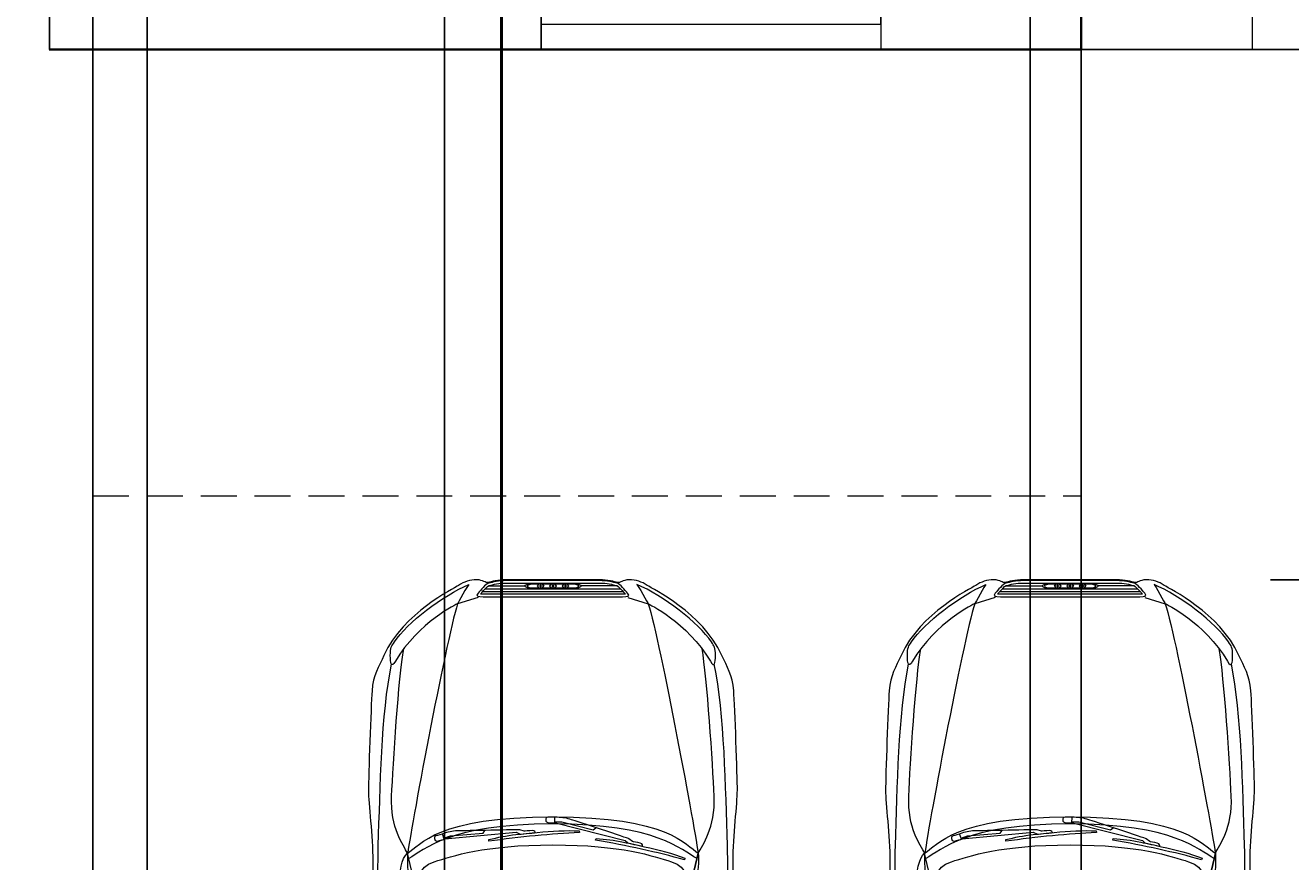
# Model space of a CAD drawing. Units: inches. Extents: x 1770 to 2988, y 1161 to 3221.
# Tile 4 of 44: x 2439 to 2663, y 1467 to 1614. Entities that reach past the tile are written whole.
import ezdxf

# ---------------------------------------------------------------- set-up
doc = ezdxf.new("R2010")
doc.units = ezdxf.units.IN
doc.linetypes.add('DASHED2', pattern=[9.525, 6.35, -3.175])
for name, color, linetype, lineweight in [('A-ANNO-DIMS', 2, 'Continuous', 18), ('A-DOOR', 4, 'Continuous', 18), ('A-GLAZ', 4, 'Continuous', 18), ('A-ROOF-OVHD', 7, 'DASHED2', 18), ('A-WALL', 7, 'Continuous', 35), ('AUDI', 8, 'Continuous', 13), ('C-SITE-PAVE', 8, 'Continuous', 18)]:
    doc.layers.add(name, color=color, linetype=linetype, lineweight=lineweight)
doc.styles.get("Standard").update_dxf_attribs({"font": 'arial.ttf'})
doc.dimstyles.get("Standard").update_dxf_attribs({"dimtxt": 0.18, "dimasz": 0.18, "dimexe": 0.18, "dimexo": 0.0625, "dimgap": 0.09, "dimtad": 0, "dimtih": 1, "dimtoh": 1, "dimdec": 4, "dimzin": 0, "dimdsep": 46, "dimtxsty": 'Standard', "dimcen": 0.09, "dimadec": 0, "dimazin": 0, "dimtfac": 1, "dimtdec": 4, "dimtofl": 0, "dimtmove": 0, "dimatfit": 3, "dimfxl": 1, "dimtolj": 1, "dimtzin": 0, "dimarcsym": 0})

# ---------------------------------------------------------------- blocks, each defined once
blk = doc.blocks.new('CAR-SEDAN-PLAN')
for points, knots in [([(35.35, 0), (11.45, 0.26), (7.98, 8.3), (6.52, 13.59), (6.52, 13.59), (5.56, 16.72), (4.79, 19.21), (4.41, 20.48), (4.41, 20.48), (4.03, 21.76), (3.2, 25.65), (3.14, 28.9), (3.14, 28.9), (3.07, 32.16), (2.76, 51.56), (2.76, 56.91), (2.76, 56.91), (2.76, 62.27), (2.76, 87.35), (2.76, 90.92), (2.76, 90.92), (2.76, 94.49), (3.52, 108.72), (3.52, 113.25), (3.52, 113.25), (3.52, 117.78), (2.76, 123.46), (2.76, 125.81), (2.76, 125.81), (2.76, 128.17), (3.2, 140.62), (3.39, 143.36), (3.39, 143.36), (3.58, 146.1), (4.61, 147.66), (5.5, 149.61), (5.5, 149.61), (8.94, 157.2), (17.74, 161.35), (18.69, 161.99), (18.69, 161.99), (19.65, 162.63), (20.67, 162.97), (21.88, 162.97), (21.88, 162.97), (23.1, 162.97), (23.41, 162.37), (23.92, 162.5), (23.92, 162.5), (24.43, 162.63), (25.7, 162.97), (27.11, 162.97), (27.11, 162.97), (28.52, 162.97), (35.35, 162.97), (35.35, 162.97), (35.35, 162.97), (35.35, 162.97), (42.18, 162.97), (43.59, 162.97), (43.59, 162.97), (45, 162.97), (46.27, 162.63), (46.78, 162.5), (46.78, 162.5), (47.29, 162.37), (47.6, 162.97), (48.82, 162.97), (48.82, 162.97), (50.04, 162.97), (51.05, 162.63), (52.01, 161.99), (52.01, 161.99), (52.96, 161.35), (61.76, 157.2), (65.21, 149.61), (65.21, 149.61), (66.09, 147.66), (67.12, 146.1), (67.31, 143.36), (67.31, 143.36), (67.5, 140.62), (67.95, 128.17), (67.95, 125.81), (67.95, 125.81), (67.95, 123.46), (67.18, 117.78), (67.18, 113.25), (67.18, 113.25), (67.18, 108.72), (67.95, 94.49), (67.95, 90.92), (67.95, 90.92), (67.95, 87.35), (67.95, 62.27), (67.95, 56.91), (67.95, 56.91), (67.95, 51.56), (67.63, 32.16), (67.57, 28.9), (67.57, 28.9), (67.5, 25.65), (66.67, 21.76), (66.29, 20.48), (66.29, 20.48), (65.91, 19.21), (65.14, 16.72), (64.19, 13.59), (64.19, 13.59), (62.72, 8.3), (59.25, 0.26), (35.35, 0)], [0, 0, 0, 0, 0.035714, 0.035714, 0.035714, 0.035714, 0.071429, 0.071429, 0.071429, 0.071429, 0.107143, 0.107143, 0.107143, 0.107143, 0.142857, 0.142857, 0.142857, 0.142857, 0.178571, 0.178571, 0.178571, 0.178571, 0.214286, 0.214286, 0.214286, 0.214286, 0.25, 0.25, 0.25, 0.25, 0.285714, 0.285714, 0.285714, 0.285714, 0.321429, 0.321429, 0.321429, 0.321429, 0.357143, 0.357143, 0.357143, 0.357143, 0.392857, 0.392857, 0.392857, 0.392857, 0.428571, 0.428571, 0.428571, 0.428571, 0.464286, 0.464286, 0.464286, 0.464286, 0.5, 0.5, 0.5, 0.5, 0.535714, 0.535714, 0.535714, 0.535714, 0.571429, 0.571429, 0.571429, 0.571429, 0.607143, 0.607143, 0.607143, 0.607143, 0.642857, 0.642857, 0.642857, 0.642857, 0.678571, 0.678571, 0.678571, 0.678571, 0.714286, 0.714286, 0.714286, 0.714286, 0.75, 0.75, 0.75, 0.75, 0.785714, 0.785714, 0.785714, 0.785714, 0.821429, 0.821429, 0.821429, 0.821429, 0.857143, 0.857143, 0.857143, 0.857143, 0.892857, 0.892857, 0.892857, 0.892857, 0.928571, 0.928571, 0.928571, 0.928571, 0.964286, 0.964286, 0.964286, 0.964286, 1, 1, 1, 1]), ([(6.62, 149.63), (6.62, 148.21), (6.78, 147.35), (7.51, 148.58), (7.51, 148.58), (11.6, 155.5), (18.51, 158.75), (18.51, 158.75), (18.51, 158.75), (18.51, 158.75), (20.38, 162.11), (20.5, 162.15), (20.5, 162.15), (15.94, 160.22), (9.53, 155.36), (7.35, 151.99), (7.35, 151.99), (6.83, 151.3), (6.62, 150.96), (6.62, 149.63)], [0, 0, 0, 0, 0.2, 0.2, 0.2, 0.2, 0.4, 0.4, 0.4, 0.4, 0.6, 0.6, 0.6, 0.6, 0.8, 0.8, 0.8, 0.8, 1, 1, 1, 1]), ([(6.62, 149.63), (6.62, 148.21), (6.78, 147.35), (7.51, 148.58), (7.51, 148.58), (11.6, 155.5), (18.51, 158.75), (18.51, 158.75), (18.51, 158.75), (18.51, 158.75), (20.38, 162.11), (20.5, 162.15), (20.5, 162.15), (15.94, 160.22), (9.53, 155.36), (7.35, 151.99), (7.35, 151.99), (6.83, 151.3), (6.62, 150.96), (6.62, 149.63)], [0, 0, 0, 0, 0.2, 0.2, 0.2, 0.2, 0.4, 0.4, 0.4, 0.4, 0.6, 0.6, 0.6, 0.6, 0.8, 0.8, 0.8, 0.8, 1, 1, 1, 1]), ([(35.49, 162.83), (35.49, 162.83), (43.59, 162.83), (43.59, 162.83), (43.59, 162.83), (44.89, 162.83), (46.07, 162.53), (46.64, 162.39), (46.64, 162.39), (46.64, 162.39), (46.74, 162.36), (46.74, 162.36), (46.74, 162.36), (47.26, 162.2), (48.06, 161.16), (48.56, 160.6), (48.56, 160.6), (49.07, 160.04), (48.56, 159.99), (47.66, 159.99), (47.66, 159.99), (46.75, 159.99), (35.35, 159.99), (35.35, 159.99), (35.35, 159.99), (35.35, 159.99), (23.95, 159.99), (23.04, 159.99), (23.04, 159.99), (22.14, 159.99), (21.63, 160.04), (22.14, 160.6), (22.14, 160.6), (22.64, 161.16), (23.44, 162.2), (23.96, 162.36), (23.96, 162.36), (23.96, 162.36), (24.06, 162.39), (24.06, 162.39), (24.06, 162.39), (24.63, 162.53), (25.81, 162.83), (27.11, 162.83), (27.11, 162.83), (27.11, 162.83), (35.22, 162.83), (35.22, 162.83), (35.22, 162.83), (35.22, 162.83), (35.49, 162.83), (35.49, 162.83)], [0, 0, 0, 0, 0.076923, 0.076923, 0.076923, 0.076923, 0.153846, 0.153846, 0.153846, 0.153846, 0.230769, 0.230769, 0.230769, 0.230769, 0.307692, 0.307692, 0.307692, 0.307692, 0.384615, 0.384615, 0.384615, 0.384615, 0.461538, 0.461538, 0.461538, 0.461538, 0.538462, 0.538462, 0.538462, 0.538462, 0.615385, 0.615385, 0.615385, 0.615385, 0.692308, 0.692308, 0.692308, 0.692308, 0.769231, 0.769231, 0.769231, 0.769231, 0.846154, 0.846154, 0.846154, 0.846154, 0.923077, 0.923077, 0.923077, 0.923077, 1, 1, 1, 1]), ([(23.04, 160.41), (23.04, 160.41), (23.04, 160.41), (23.04, 160.41), (23.04, 160.41), (23.04, 160.41), (47.66, 160.41), (47.66, 160.41), (47.66, 160.41), (47.87, 160.41), (48.03, 160.42), (48.16, 160.43), (48.16, 160.43), (48.06, 160.54), (47.9, 160.72), (47.9, 160.72), (47.9, 160.72), (47.53, 161.15), (46.91, 161.87), (46.62, 161.96), (46.62, 161.96), (46.62, 161.96), (46.53, 161.98), (46.53, 161.98), (46.53, 161.98), (45.98, 162.12), (44.84, 162.41), (43.59, 162.41), (43.59, 162.41), (43.59, 162.41), (27.11, 162.41), (27.11, 162.41), (27.11, 162.41), (25.87, 162.41), (24.72, 162.12), (24.17, 161.98), (24.17, 161.98), (24.17, 161.98), (24.06, 161.95), (24.06, 161.95), (24.06, 161.95), (23.79, 161.87), (23.17, 161.15), (22.8, 160.72), (22.8, 160.72), (22.8, 160.72), (22.65, 160.54), (22.55, 160.43), (22.55, 160.43), (22.68, 160.42), (22.84, 160.41), (23.04, 160.41)], [0, 0, 0, 0, 0.076923, 0.076923, 0.076923, 0.076923, 0.153846, 0.153846, 0.153846, 0.153846, 0.230769, 0.230769, 0.230769, 0.230769, 0.307692, 0.307692, 0.307692, 0.307692, 0.384615, 0.384615, 0.384615, 0.384615, 0.461538, 0.461538, 0.461538, 0.461538, 0.538462, 0.538462, 0.538462, 0.538462, 0.615385, 0.615385, 0.615385, 0.615385, 0.692308, 0.692308, 0.692308, 0.692308, 0.769231, 0.769231, 0.769231, 0.769231, 0.846154, 0.846154, 0.846154, 0.846154, 0.923077, 0.923077, 0.923077, 0.923077, 1, 1, 1, 1]), ([(32.06, 161.44), (32.49, 161.44), (32.87, 161.48), (33.16, 161.56), (33.16, 161.56), (33.46, 161.48), (33.86, 161.44), (34.29, 161.44), (34.29, 161.44), (34.72, 161.44), (35.09, 161.48), (35.39, 161.55), (35.39, 161.55), (35.65, 161.48), (36.06, 161.44), (36.46, 161.44), (36.46, 161.44), (36.89, 161.44), (37.29, 161.48), (37.58, 161.56), (37.58, 161.56), (37.88, 161.48), (38.25, 161.44), (38.68, 161.44), (38.68, 161.44), (39.59, 161.44), (40.34, 161.64), (40.34, 161.88), (40.34, 161.88), (40.34, 162.12), (39.59, 162.32), (38.68, 162.32), (38.68, 162.32), (38.25, 162.32), (37.88, 162.27), (37.58, 162.21), (37.58, 162.21), (37.29, 162.27), (36.89, 162.32), (36.46, 162.32), (36.46, 162.32), (36.06, 162.32), (35.65, 162.28), (35.39, 162.21), (35.39, 162.21), (35.09, 162.28), (34.72, 162.32), (34.29, 162.32), (34.29, 162.32), (33.81, 162.32), (33.29, 162.24), (33.16, 162.21), (33.16, 162.21), (32.87, 162.27), (32.49, 162.32), (32.06, 162.32), (32.06, 162.32), (31.15, 162.32), (30.4, 162.12), (30.4, 161.88), (30.4, 161.88), (30.4, 161.64), (31.15, 161.44), (32.06, 161.44)], [0, 0, 0, 0, 0.0625, 0.0625, 0.0625, 0.0625, 0.125, 0.125, 0.125, 0.125, 0.1875, 0.1875, 0.1875, 0.1875, 0.25, 0.25, 0.25, 0.25, 0.3125, 0.3125, 0.3125, 0.3125, 0.375, 0.375, 0.375, 0.375, 0.4375, 0.4375, 0.4375, 0.4375, 0.5, 0.5, 0.5, 0.5, 0.5625, 0.5625, 0.5625, 0.5625, 0.625, 0.625, 0.625, 0.625, 0.6875, 0.6875, 0.6875, 0.6875, 0.75, 0.75, 0.75, 0.75, 0.8125, 0.8125, 0.8125, 0.8125, 0.875, 0.875, 0.875, 0.875, 0.9375, 0.9375, 0.9375, 0.9375, 1, 1, 1, 1]), ([(32.06, 161.44), (32.49, 161.44), (32.87, 161.48), (33.16, 161.56), (33.16, 161.56), (33.46, 161.48), (33.86, 161.44), (34.29, 161.44), (34.29, 161.44), (34.72, 161.44), (35.09, 161.48), (35.39, 161.55), (35.39, 161.55), (35.65, 161.48), (36.06, 161.44), (36.46, 161.44), (36.46, 161.44), (36.89, 161.44), (37.29, 161.48), (37.58, 161.56), (37.58, 161.56), (37.88, 161.48), (38.25, 161.44), (38.68, 161.44), (38.68, 161.44), (39.59, 161.44), (40.34, 161.64), (40.34, 161.88), (40.34, 161.88), (40.34, 162.12), (39.59, 162.32), (38.68, 162.32), (38.68, 162.32), (38.25, 162.32), (37.88, 162.27), (37.58, 162.21), (37.58, 162.21), (37.29, 162.27), (36.89, 162.32), (36.46, 162.32), (36.46, 162.32), (36.06, 162.32), (35.65, 162.28), (35.39, 162.21), (35.39, 162.21), (35.09, 162.28), (34.72, 162.32), (34.29, 162.32), (34.29, 162.32), (33.81, 162.32), (33.29, 162.24), (33.16, 162.21), (33.16, 162.21), (32.87, 162.27), (32.49, 162.32), (32.06, 162.32), (32.06, 162.32), (31.15, 162.32), (30.4, 162.12), (30.4, 161.88), (30.4, 161.88), (30.4, 161.64), (31.15, 161.44), (32.06, 161.44)], [0, 0, 0, 0, 0.0625, 0.0625, 0.0625, 0.0625, 0.125, 0.125, 0.125, 0.125, 0.1875, 0.1875, 0.1875, 0.1875, 0.25, 0.25, 0.25, 0.25, 0.3125, 0.3125, 0.3125, 0.3125, 0.375, 0.375, 0.375, 0.375, 0.4375, 0.4375, 0.4375, 0.4375, 0.5, 0.5, 0.5, 0.5, 0.5625, 0.5625, 0.5625, 0.5625, 0.625, 0.625, 0.625, 0.625, 0.6875, 0.6875, 0.6875, 0.6875, 0.75, 0.75, 0.75, 0.75, 0.8125, 0.8125, 0.8125, 0.8125, 0.875, 0.875, 0.875, 0.875, 0.9375, 0.9375, 0.9375, 0.9375, 1, 1, 1, 1]), ([(32.06, 162.21), (32.39, 162.21), (32.68, 162.18), (32.89, 162.12), (32.89, 162.12), (32.73, 162.05), (32.63, 161.97), (32.63, 161.88), (32.63, 161.88), (32.63, 161.79), (32.73, 161.71), (32.89, 161.64), (32.89, 161.64), (32.68, 161.59), (32.39, 161.55), (32.06, 161.55), (32.06, 161.55), (31.37, 161.55), (30.83, 161.69), (30.83, 161.88), (30.83, 161.88), (30.83, 162.06), (31.37, 162.21), (32.06, 162.21)], [0, 0, 0, 0, 0.166667, 0.166667, 0.166667, 0.166667, 0.333333, 0.333333, 0.333333, 0.333333, 0.5, 0.5, 0.5, 0.5, 0.666667, 0.666667, 0.666667, 0.666667, 0.833333, 0.833333, 0.833333, 0.833333, 1, 1, 1, 1]), ([(33.3, 161.88), (33.3, 161.82), (33.24, 161.78), (33.16, 161.74), (33.16, 161.74), (33.08, 161.78), (33.06, 161.82), (33.06, 161.88), (33.06, 161.88), (33.06, 161.93), (33.08, 161.98), (33.16, 162.03), (33.16, 162.03), (33.24, 161.98), (33.3, 161.93), (33.3, 161.88)], [0, 0, 0, 0, 0.25, 0.25, 0.25, 0.25, 0.5, 0.5, 0.5, 0.5, 0.75, 0.75, 0.75, 0.75, 1, 1, 1, 1]), ([(35.09, 162.13), (34.93, 162.06), (34.82, 161.97), (34.82, 161.88), (34.82, 161.88), (34.82, 161.79), (34.93, 161.7), (35.09, 161.63), (35.09, 161.63), (34.88, 161.58), (34.61, 161.55), (34.29, 161.55), (34.29, 161.55), (33.97, 161.55), (33.67, 161.59), (33.46, 161.64), (33.46, 161.64), (33.62, 161.71), (33.73, 161.79), (33.73, 161.88), (33.73, 161.88), (33.73, 161.97), (33.62, 162.05), (33.46, 162.12), (33.46, 162.12), (33.67, 162.18), (33.97, 162.21), (34.29, 162.21), (34.29, 162.21), (34.61, 162.21), (34.88, 162.18), (35.09, 162.13)], [0, 0, 0, 0, 0.125, 0.125, 0.125, 0.125, 0.25, 0.25, 0.25, 0.25, 0.375, 0.375, 0.375, 0.375, 0.5, 0.5, 0.5, 0.5, 0.625, 0.625, 0.625, 0.625, 0.75, 0.75, 0.75, 0.75, 0.875, 0.875, 0.875, 0.875, 1, 1, 1, 1]), ([(35.52, 161.88), (35.52, 161.82), (35.47, 161.77), (35.39, 161.72), (35.39, 161.72), (35.28, 161.77), (35.23, 161.82), (35.23, 161.88), (35.23, 161.88), (35.23, 161.93), (35.28, 161.99), (35.39, 162.03), (35.39, 162.03), (35.47, 161.99), (35.52, 161.93), (35.52, 161.88)], [0, 0, 0, 0, 0.25, 0.25, 0.25, 0.25, 0.5, 0.5, 0.5, 0.5, 0.75, 0.75, 0.75, 0.75, 1, 1, 1, 1]), ([(37.32, 162.12), (37.13, 162.05), (37.02, 161.97), (37.02, 161.88), (37.02, 161.88), (37.02, 161.79), (37.13, 161.71), (37.32, 161.64), (37.32, 161.64), (37.07, 161.59), (36.78, 161.55), (36.46, 161.55), (36.46, 161.55), (36.16, 161.55), (35.87, 161.58), (35.65, 161.63), (35.65, 161.63), (35.84, 161.7), (35.95, 161.79), (35.95, 161.88), (35.95, 161.88), (35.95, 161.97), (35.84, 162.06), (35.65, 162.13), (35.65, 162.13), (35.87, 162.18), (36.16, 162.21), (36.46, 162.21), (36.46, 162.21), (36.78, 162.21), (37.07, 162.18), (37.32, 162.12)], [0, 0, 0, 0, 0.125, 0.125, 0.125, 0.125, 0.25, 0.25, 0.25, 0.25, 0.375, 0.375, 0.375, 0.375, 0.5, 0.5, 0.5, 0.5, 0.625, 0.625, 0.625, 0.625, 0.75, 0.75, 0.75, 0.75, 0.875, 0.875, 0.875, 0.875, 1, 1, 1, 1]), ([(37.72, 161.88), (37.72, 161.82), (37.66, 161.78), (37.58, 161.74), (37.58, 161.74), (37.5, 161.78), (37.45, 161.82), (37.45, 161.88), (37.45, 161.88), (37.45, 161.93), (37.5, 161.98), (37.58, 162.03), (37.58, 162.03), (37.66, 161.98), (37.72, 161.93), (37.72, 161.88)], [0, 0, 0, 0, 0.25, 0.25, 0.25, 0.25, 0.5, 0.5, 0.5, 0.5, 0.75, 0.75, 0.75, 0.75, 1, 1, 1, 1]), ([(39.91, 161.88), (39.91, 161.69), (39.38, 161.55), (38.68, 161.55), (38.68, 161.55), (38.36, 161.55), (38.07, 161.59), (37.85, 161.64), (37.85, 161.64), (38.01, 161.71), (38.12, 161.79), (38.12, 161.88), (38.12, 161.88), (38.12, 161.97), (38.01, 162.05), (37.85, 162.12), (37.85, 162.12), (38.07, 162.18), (38.36, 162.21), (38.68, 162.21), (38.68, 162.21), (39.38, 162.21), (39.91, 162.06), (39.91, 161.88)], [0, 0, 0, 0, 0.166667, 0.166667, 0.166667, 0.166667, 0.333333, 0.333333, 0.333333, 0.333333, 0.5, 0.5, 0.5, 0.5, 0.666667, 0.666667, 0.666667, 0.666667, 0.833333, 0.833333, 0.833333, 0.833333, 1, 1, 1, 1]), ([(64.08, 149.63), (64.08, 148.21), (63.92, 147.35), (63.19, 148.58), (63.19, 148.58), (59.11, 155.5), (52.19, 158.75), (52.19, 158.75), (52.19, 158.75), (52.19, 158.75), (50.32, 162.11), (50.2, 162.15), (50.2, 162.15), (54.76, 160.22), (61.17, 155.36), (63.35, 151.99), (63.35, 151.99), (63.87, 151.3), (64.08, 150.96), (64.08, 149.63)], [0, 0, 0, 0, 0.2, 0.2, 0.2, 0.2, 0.4, 0.4, 0.4, 0.4, 0.6, 0.6, 0.6, 0.6, 0.8, 0.8, 0.8, 0.8, 1, 1, 1, 1]), ([(64.08, 149.63), (64.08, 148.21), (63.92, 147.35), (63.19, 148.58), (63.19, 148.58), (59.11, 155.5), (52.19, 158.75), (52.19, 158.75), (52.19, 158.75), (52.19, 158.75), (50.32, 162.11), (50.2, 162.15), (50.2, 162.15), (54.76, 160.22), (61.17, 155.36), (63.35, 151.99), (63.35, 151.99), (63.87, 151.3), (64.08, 150.96), (64.08, 149.63)], [0, 0, 0, 0, 0.2, 0.2, 0.2, 0.2, 0.4, 0.4, 0.4, 0.4, 0.6, 0.6, 0.6, 0.6, 0.8, 0.8, 0.8, 0.8, 1, 1, 1, 1]), ([(9.66, 114.67), (8.92, 116.16), (6.61, 119.13), (6.86, 124.74), (6.86, 124.74), (7.1, 130.36), (8.1, 145.86), (8.99, 150.79)], [0, 0, 0, 0, 0.5, 0.5, 0.5, 0.5, 1, 1, 1, 1]), ([(61.04, 114.67), (61.78, 116.16), (64.09, 119.13), (63.85, 124.74), (63.85, 124.74), (63.6, 130.36), (62.6, 145.86), (61.71, 150.79)], [0, 0, 0, 0, 0.5, 0.5, 0.5, 0.5, 1, 1, 1, 1]), ([(7.64, 13.52), (6.44, 19.53), (5.16, 31.7), (4.94, 44.37), (4.94, 44.37), (4.72, 57.04), (4.17, 105.75), (4.5, 116.02), (4.5, 116.02), (4.83, 126.28), (5.01, 139.24), (6.83, 148.05)], [0, 0, 0, 0, 0.333333, 0.333333, 0.333333, 0.333333, 0.666667, 0.666667, 0.666667, 0.666667, 1, 1, 1, 1]), ([(63.07, 13.52), (64.27, 19.53), (65.54, 31.7), (65.76, 44.37), (65.76, 44.37), (65.98, 57.04), (66.53, 105.75), (66.2, 116.02), (66.2, 116.02), (65.87, 126.28), (65.69, 139.24), (63.87, 148.05)], [0, 0, 0, 0, 0.333333, 0.333333, 0.333333, 0.333333, 0.666667, 0.666667, 0.666667, 0.666667, 1, 1, 1, 1]), ([(35.35, 92.33), (46.17, 92.33), (55.33, 90.37), (55.33, 90.37), (55.33, 90.37), (55.33, 90.37), (61.04, 114.67), (61.04, 114.67), (61.04, 114.67), (58.76, 116.14), (55.78, 121.11), (35.35, 121.11), (35.35, 121.11), (14.92, 121.11), (11.94, 116.14), (9.66, 114.67), (9.66, 114.67), (9.66, 114.67), (15.37, 90.37), (15.37, 90.37), (15.37, 90.37), (15.37, 90.37), (24.53, 92.33), (35.35, 92.33)], [0, 0, 0, 0, 0.166667, 0.166667, 0.166667, 0.166667, 0.333333, 0.333333, 0.333333, 0.333333, 0.5, 0.5, 0.5, 0.5, 0.666667, 0.666667, 0.666667, 0.666667, 0.833333, 0.833333, 0.833333, 0.833333, 1, 1, 1, 1]), ([(35.35, 92.33), (46.17, 92.33), (55.33, 90.37), (55.33, 90.37), (55.33, 90.37), (55.33, 90.37), (61.04, 114.67), (61.04, 114.67), (61.04, 114.67), (58.76, 116.14), (55.78, 121.11), (35.35, 121.11), (35.35, 121.11), (14.92, 121.11), (11.94, 116.14), (9.66, 114.67), (9.66, 114.67), (9.66, 114.67), (15.37, 90.37), (15.37, 90.37), (15.37, 90.37), (15.37, 90.37), (24.53, 92.33), (35.35, 92.33)], [0, 0, 0, 0, 0.166667, 0.166667, 0.166667, 0.166667, 0.333333, 0.333333, 0.333333, 0.333333, 0.5, 0.5, 0.5, 0.5, 0.666667, 0.666667, 0.666667, 0.666667, 0.833333, 0.833333, 0.833333, 0.833333, 1, 1, 1, 1]), ([(36.09, 121.02), (37.08, 121.02), (37.81, 120.86), (38.66, 120.59), (38.66, 120.59), (39.31, 120.41), (48.79, 117.24), (48.79, 117.24), (48.79, 117.24), (48.79, 117.24), (49.43, 116.73), (49.43, 116.73), (49.43, 116.73), (49.43, 116.73), (50.29, 116.57), (50.77, 116.47), (50.77, 116.47), (51.26, 116.33), (51.2, 115.9), (51.2, 115.9), (51.2, 115.9), (51.2, 115.9), (48.58, 116.49), (48.58, 116.49), (48.58, 116.49), (48.58, 116.49), (48.15, 116.92), (48.15, 116.92), (48.15, 116.92), (48.15, 116.92), (35.82, 120.06), (35.82, 120.06), (35.82, 120.06), (35.82, 120.06), (35.42, 120.06), (34.8, 120.06), (34.8, 120.06), (34.19, 120.09), (34.08, 120.3), (34.08, 120.54), (34.08, 120.54), (34.08, 120.81), (34.11, 121.05), (34.48, 121.05), (34.48, 121.05), (34.86, 121.08), (35.47, 121.05), (36.09, 121.02)], [0, 0, 0, 0, 0.083333, 0.083333, 0.083333, 0.083333, 0.166667, 0.166667, 0.166667, 0.166667, 0.25, 0.25, 0.25, 0.25, 0.333333, 0.333333, 0.333333, 0.333333, 0.416667, 0.416667, 0.416667, 0.416667, 0.5, 0.5, 0.5, 0.5, 0.583333, 0.583333, 0.583333, 0.583333, 0.666667, 0.666667, 0.666667, 0.666667, 0.75, 0.75, 0.75, 0.75, 0.833333, 0.833333, 0.833333, 0.833333, 0.916667, 0.916667, 0.916667, 0.916667, 1, 1, 1, 1]), ([(60.82, 113.75), (58.05, 115.23), (53.75, 119.85), (35.35, 119.85), (35.35, 119.85), (16.95, 119.85), (12.66, 115.23), (9.88, 113.75)], [0, 0, 0, 0, 0.5, 0.5, 0.5, 0.5, 1, 1, 1, 1]), ([(16.21, 118.21), (17.12, 118.53), (17.87, 118.61), (18.78, 118.64), (18.78, 118.64), (19.45, 118.64), (29.53, 118.83), (29.53, 118.83), (29.53, 118.83), (29.53, 118.83), (30.3, 118.56), (30.3, 118.56), (30.3, 118.56), (30.3, 118.56), (31.19, 118.66), (31.67, 118.69), (31.67, 118.69), (32.15, 118.75), (32.23, 118.32), (32.23, 118.32), (32.23, 118.32), (32.23, 118.32), (29.58, 118.05), (29.58, 118.05), (29.58, 118.05), (29.58, 118.05), (28.86, 118.4), (28.86, 118.4), (28.86, 118.4), (28.86, 118.4), (16.26, 117.22), (16.26, 117.22), (16.26, 117.22), (16.26, 117.22), (15.89, 117.08), (15.3, 116.9), (15.3, 116.9), (14.74, 116.71), (14.55, 116.87), (14.47, 117.11), (14.47, 117.11), (14.39, 117.38), (14.33, 117.59), (14.68, 117.73), (14.68, 117.73), (15.03, 117.83), (15.62, 118.02), (16.21, 118.21)], [0, 0, 0, 0, 0.083333, 0.083333, 0.083333, 0.083333, 0.166667, 0.166667, 0.166667, 0.166667, 0.25, 0.25, 0.25, 0.25, 0.333333, 0.333333, 0.333333, 0.333333, 0.416667, 0.416667, 0.416667, 0.416667, 0.5, 0.5, 0.5, 0.5, 0.583333, 0.583333, 0.583333, 0.583333, 0.666667, 0.666667, 0.666667, 0.666667, 0.75, 0.75, 0.75, 0.75, 0.833333, 0.833333, 0.833333, 0.833333, 0.916667, 0.916667, 0.916667, 0.916667, 1, 1, 1, 1]), ([(16.21, 118.21), (17.12, 118.53), (17.87, 118.61), (18.78, 118.64), (18.78, 118.64), (19.45, 118.64), (29.53, 118.83), (29.53, 118.83), (29.53, 118.83), (29.53, 118.83), (30.3, 118.56), (30.3, 118.56), (30.3, 118.56), (30.3, 118.56), (31.19, 118.66), (31.67, 118.69), (31.67, 118.69), (32.15, 118.75), (32.23, 118.32), (32.23, 118.32), (32.23, 118.32), (32.23, 118.32), (29.58, 118.05), (29.58, 118.05), (29.58, 118.05), (29.58, 118.05), (28.86, 118.4), (28.86, 118.4), (28.86, 118.4), (28.86, 118.4), (16.26, 117.22), (16.26, 117.22), (16.26, 117.22), (16.26, 117.22), (15.89, 117.08), (15.3, 116.9), (15.3, 116.9), (14.74, 116.71), (14.55, 116.87), (14.47, 117.11), (14.47, 117.11), (14.39, 117.38), (14.33, 117.59), (14.68, 117.73), (14.68, 117.73), (15.03, 117.83), (15.62, 118.02), (16.21, 118.21)], [0, 0, 0, 0, 0.083333, 0.083333, 0.083333, 0.083333, 0.166667, 0.166667, 0.166667, 0.166667, 0.25, 0.25, 0.25, 0.25, 0.333333, 0.333333, 0.333333, 0.333333, 0.416667, 0.416667, 0.416667, 0.416667, 0.5, 0.5, 0.5, 0.5, 0.583333, 0.583333, 0.583333, 0.583333, 0.666667, 0.666667, 0.666667, 0.666667, 0.75, 0.75, 0.75, 0.75, 0.833333, 0.833333, 0.833333, 0.833333, 0.916667, 0.916667, 0.916667, 0.916667, 1, 1, 1, 1]), ([(16.1, 117.35), (16.1, 117.35), (17.26, 117.73), (17.26, 117.73), (17.26, 117.73), (17.26, 117.73), (23.02, 118.24), (23.02, 118.24), (23.02, 118.24), (23.02, 118.24), (23.34, 118.69), (23.34, 118.69)], [0, 0, 0, 0, 0.333333, 0.333333, 0.333333, 0.333333, 0.666667, 0.666667, 0.666667, 0.666667, 1, 1, 1, 1]), ([(40, 118.61), (37.7, 118.77), (35.18, 118.58), (32.58, 118.34), (32.58, 118.34), (31.32, 118.21), (30.06, 118.1), (28.83, 117.97), (28.83, 117.97), (27.09, 117.81), (25.61, 117.46), (24.01, 117.08), (24.01, 117.08), (24.01, 117.08), (24.01, 116.79), (24.01, 116.79), (24.01, 116.79), (29.47, 117.57), (35.15, 118.1), (40.03, 118.32), (40.03, 118.32), (40.03, 118.32), (40, 118.61), (40, 118.61)], [0, 0, 0, 0, 0.166667, 0.166667, 0.166667, 0.166667, 0.333333, 0.333333, 0.333333, 0.333333, 0.5, 0.5, 0.5, 0.5, 0.666667, 0.666667, 0.666667, 0.666667, 0.833333, 0.833333, 0.833333, 0.833333, 1, 1, 1, 1]), ([(35.69, 120.25), (35.69, 120.25), (36.92, 120.22), (36.92, 120.22), (36.92, 120.22), (36.92, 120.22), (42.49, 118.83), (42.49, 118.83), (42.49, 118.83), (42.49, 118.83), (42.95, 119.17), (42.95, 119.17)], [0, 0, 0, 0, 0.333333, 0.333333, 0.333333, 0.333333, 0.666667, 0.666667, 0.666667, 0.666667, 1, 1, 1, 1]), ([(58.68, 113.81), (56.53, 114.64), (54.1, 115.26), (51.52, 115.82), (51.52, 115.82), (50.29, 116.09), (49.06, 116.39), (47.85, 116.63), (47.85, 116.63), (46.17, 117), (44.64, 117.14), (42.98, 117.27), (42.98, 117.27), (42.98, 117.27), (42.9, 117), (42.9, 117), (42.9, 117), (48.34, 116.06), (53.88, 114.83), (58.6, 113.52), (58.6, 113.52), (58.6, 113.52), (58.68, 113.81), (58.68, 113.81)], [0, 0, 0, 0, 0.166667, 0.166667, 0.166667, 0.166667, 0.333333, 0.333333, 0.333333, 0.333333, 0.5, 0.5, 0.5, 0.5, 0.666667, 0.666667, 0.666667, 0.666667, 0.833333, 0.833333, 0.833333, 0.833333, 1, 1, 1, 1]), ([(9.66, 114.67), (9.66, 114.67), (15.37, 90.37), (15.37, 90.37), (15.37, 90.37), (15.37, 90.37), (14.48, 91.26), (14.15, 92.64), (14.15, 92.64), (13.82, 94.03), (10.04, 109.86), (9.79, 111.17), (9.79, 111.17), (9.55, 112.47), (9.66, 114.67), (9.66, 114.67)], [0, 0, 0, 0, 0.25, 0.25, 0.25, 0.25, 0.5, 0.5, 0.5, 0.5, 0.75, 0.75, 0.75, 0.75, 1, 1, 1, 1]), ([(9.66, 114.67), (9.66, 114.67), (15.37, 90.37), (15.37, 90.37), (15.37, 90.37), (15.37, 90.37), (14.48, 91.26), (14.15, 92.64), (14.15, 92.64), (13.82, 94.03), (10.04, 109.86), (9.79, 111.17), (9.79, 111.17), (9.55, 112.47), (9.66, 114.67), (9.66, 114.67)], [0, 0, 0, 0, 0.25, 0.25, 0.25, 0.25, 0.5, 0.5, 0.5, 0.5, 0.75, 0.75, 0.75, 0.75, 1, 1, 1, 1]), ([(35.35, 93.86), (43.94, 93.86), (50.97, 92.45), (52.59, 92.2), (52.59, 92.2), (53.92, 92), (55.15, 93.44), (55.52, 95.16), (55.52, 95.16), (55.89, 96.88), (58.26, 106.94), (58.59, 108.38), (58.59, 108.38), (58.92, 109.82), (59.47, 112.19), (56.31, 113.17), (56.31, 113.17), (53.15, 114.15), (47.56, 116.15), (35.35, 116.15), (35.35, 116.15), (23.15, 116.15), (17.55, 114.15), (14.39, 113.17), (14.39, 113.17), (11.23, 112.19), (11.79, 109.82), (12.11, 108.38), (12.11, 108.38), (12.44, 106.94), (14.81, 96.88), (15.18, 95.16), (15.18, 95.16), (15.55, 93.44), (16.78, 92), (18.11, 92.2), (18.11, 92.2), (19.74, 92.45), (26.76, 93.86), (35.35, 93.86)], [0, 0, 0, 0, 0.1, 0.1, 0.1, 0.1, 0.2, 0.2, 0.2, 0.2, 0.3, 0.3, 0.3, 0.3, 0.4, 0.4, 0.4, 0.4, 0.5, 0.5, 0.5, 0.5, 0.6, 0.6, 0.6, 0.6, 0.7, 0.7, 0.7, 0.7, 0.8, 0.8, 0.8, 0.8, 0.9, 0.9, 0.9, 0.9, 1, 1, 1, 1]), ([(61.04, 114.67), (61.04, 114.67), (55.33, 90.37), (55.33, 90.37), (55.33, 90.37), (55.33, 90.37), (56.23, 91.26), (56.55, 92.64), (56.55, 92.64), (56.88, 94.03), (60.66, 109.86), (60.91, 111.17), (60.91, 111.17), (61.15, 112.47), (61.04, 114.67), (61.04, 114.67)], [0, 0, 0, 0, 0.25, 0.25, 0.25, 0.25, 0.5, 0.5, 0.5, 0.5, 0.75, 0.75, 0.75, 0.75, 1, 1, 1, 1])]:
    blk.add_open_spline(points, degree=3, knots=knots)
for points in [[(23.41, 161.4), (23.41, 161.4), (47.23, 161.4), (47.23, 161.4)], [(23.96, 161.9), (23.96, 161.9), (30.4, 161.9), (30.4, 161.9)], [(46.75, 161.9), (46.75, 161.9), (40.3, 161.9), (40.3, 161.9)], [(22.13, 159.86), (22.13, 159.86), (18.51, 158.75), (18.51, 158.75)], [(22.94, 160.88), (22.94, 160.88), (47.74, 160.88), (47.74, 160.88)], [(48.57, 159.86), (48.57, 159.86), (52.19, 158.75), (52.19, 158.75)], [(18.51, 158.75), (16.41, 152.05), (10.02, 117.73), (9.65, 114.38)], [(52.19, 158.75), (54.3, 152.05), (60.68, 117.73), (61.05, 114.38)], [(35.69, 120.06), (35.69, 120.06), (35.72, 121.05), (35.72, 121.05)], [(16.16, 117.16), (16.16, 117.16), (15.83, 118.1), (15.83, 118.1)], [(8.16, 109.91), (8.28, 111.03), (8.55, 113.81), (9.66, 114.67)]]:
    blk.add_open_spline(points, degree=3)
blk = doc.blocks.new('WIN-60-EXT')
for p, q in [((0, 9), (0, 0)), ((60, 4.5), (60, 9)), ((60, 9), (60, 0)), ((0, 0), (0, 4.5)), ((0, 4.5), (60, 4.5))]:
    blk.add_line(p, q)
blk = doc.blocks.new('*D50')
at = {"layer": 'A-ANNO-DIMS', "color": 0, "lineweight": -2, "transparency": 16777216}
for p, q in [((2659.16, 1516.52), (2683.72, 1516.52)), ((2683.54, 1516.34), (2683.54, 1435.22)), ((2683.54, 1353.73), (2683.54, 1434.85)), ((2659.16, 1353.55), (2683.72, 1353.55))]:
    blk.add_line(p, q, dxfattribs=at)
at = {"layer": 'A-ANNO-DIMS', "color": 0, "transparency": 16777216}
for points in [[(2683.51, 1516.34), (2683.57, 1516.34), (2683.54, 1516.52)], [(2683.51, 1353.73), (2683.57, 1353.73), (2683.54, 1353.55)]]:
    blk.add_solid(points, dxfattribs=at)
at = {"layer": 'Defpoints', "color": 0, "transparency": 16777216}
for p in [(2659.1, 1516.52), (2683.54, 1516.52), (2659.1, 1353.55)]:
    blk.add_point(p, dxfattribs=at)
at = {"layer": 'A-ANNO-DIMS', "color": 0, "transparency": 16777216, "insert": (2683.54, 1435.04), "char_height": 0.18, "attachment_point": 5}
blk.add_mtext('\\A1;SEDAN 163 TYP.', dxfattribs=at)
blk = doc.blocks.new('*D60')
at = {"layer": 'A-ANNO-DIMS', "color": 0, "lineweight": -2, "transparency": 16777216}
for p, q in [((2151.7, 1610.14), (2151.7, 1165.57)), ((2625.7, 1610.14), (2625.7, 1165.57)), ((2151.88, 1165.75), (2388.4, 1165.75)), ((2625.52, 1165.75), (2388.99, 1165.75))]:
    blk.add_line(p, q, dxfattribs=at)
at = {"layer": 'A-ANNO-DIMS', "color": 0, "transparency": 16777216}
for points in [[(2151.88, 1165.78), (2151.88, 1165.72), (2151.7, 1165.75)], [(2625.52, 1165.78), (2625.52, 1165.72), (2625.7, 1165.75)]]:
    blk.add_solid(points, dxfattribs=at)
at = {"layer": 'Defpoints', "color": 0, "transparency": 16777216}
for p in [(2151.7, 1610.2), (2625.7, 1610.2), (2625.7, 1165.75)]:
    blk.add_point(p, dxfattribs=at)
at = {"layer": 'A-ANNO-DIMS', "color": 0, "transparency": 16777216, "insert": (2388.7, 1165.75), "char_height": 0.18, "attachment_point": 5}
blk.add_mtext('\\A1;474', dxfattribs=at)
blk = doc.blocks.new('*D61')
at = {"layer": 'A-ANNO-DIMS', "color": 0, "lineweight": -2, "transparency": 16777216}
for p, q in [((2625.76, 2376.7), (2866.87, 2376.7)), ((2866.69, 2376.52), (2866.69, 1993.63)), ((2866.69, 1610.38), (2866.69, 1993.27)), ((2625.76, 1610.2), (2866.87, 1610.2))]:
    blk.add_line(p, q, dxfattribs=at)
at = {"layer": 'A-ANNO-DIMS', "color": 0, "transparency": 16777216}
for points in [[(2866.66, 2376.52), (2866.72, 2376.52), (2866.69, 2376.7)], [(2866.66, 1610.38), (2866.72, 1610.38), (2866.69, 1610.2)]]:
    blk.add_solid(points, dxfattribs=at)
at = {"layer": 'Defpoints', "color": 0, "transparency": 16777216}
for p in [(2625.7, 2376.7), (2866.69, 2376.7), (2625.7, 1610.2)]:
    blk.add_point(p, dxfattribs=at)
at = {"layer": 'A-ANNO-DIMS', "color": 0, "transparency": 16777216, "insert": (2866.69, 1993.45), "char_height": 0.18, "attachment_point": 5}
blk.add_mtext('\\A1;766.5', dxfattribs=at)
blk = doc.blocks.new('*D63')
at = {"layer": 'A-ANNO-DIMS', "color": 0, "lineweight": -2, "transparency": 16777216}
for p, q in [((2352.17, 1323.59), (2352.17, 2570.7)), ((2352.35, 2570.52), (2401.24, 2570.52)), ((2450.91, 2570.52), (2402.02, 2570.52)), ((2451.09, 1323.59), (2451.09, 2570.7))]:
    blk.add_line(p, q, dxfattribs=at)
at = {"layer": 'A-ANNO-DIMS', "color": 0, "transparency": 16777216}
for points in [[(2352.35, 2570.55), (2352.35, 2570.49), (2352.17, 2570.52)], [(2450.91, 2570.55), (2450.91, 2570.49), (2451.09, 2570.52)]]:
    blk.add_solid(points, dxfattribs=at)
at = {"layer": 'Defpoints', "color": 0, "transparency": 16777216}
for p in [(2451.09, 2570.52), (2352.17, 1323.53), (2451.09, 1323.53)]:
    blk.add_point(p, dxfattribs=at)
at = {"layer": 'A-ANNO-DIMS', "color": 0, "transparency": 16777216, "insert": (2401.63, 2570.52), "char_height": 0.18, "attachment_point": 5}
blk.add_mtext('\\A1;98.93', dxfattribs=at)
blk = doc.blocks.new('*D74')
at = {"layer": 'A-ANNO-DIMS', "color": 0, "lineweight": -2, "transparency": 16777216}
for p, q in [((2523.42, 2097.48), (2523.42, 1165.57)), ((2616.7, 2097.48), (2616.7, 1165.57)), ((2523.6, 1165.75), (2569.66, 1165.75)), ((2616.52, 1165.75), (2570.45, 1165.75))]:
    blk.add_line(p, q, dxfattribs=at)
at = {"layer": 'A-ANNO-DIMS', "color": 0, "transparency": 16777216}
for points in [[(2523.6, 1165.78), (2523.6, 1165.72), (2523.42, 1165.75)], [(2616.52, 1165.78), (2616.52, 1165.72), (2616.7, 1165.75)]]:
    blk.add_solid(points, dxfattribs=at)
at = {"layer": 'Defpoints', "color": 0, "transparency": 16777216}
for p in [(2523.42, 2097.54), (2616.7, 2097.54), (2616.7, 1165.75)]:
    blk.add_point(p, dxfattribs=at)
at = {"layer": 'A-ANNO-DIMS', "color": 0, "transparency": 16777216, "insert": (2570.06, 1165.75), "char_height": 0.18, "attachment_point": 5}
blk.add_mtext('\\A1;93.28', dxfattribs=at)
blk = doc.blocks.new('*D77')
at = {"layer": 'A-ANNO-DIMS', "color": 0, "lineweight": -2, "transparency": 16777216}
for p, q in [((2460.7, 1710.64), (2460.7, 1165.57)), ((2616.7, 1710.64), (2616.7, 1165.57)), ((2460.88, 1165.75), (2538.42, 1165.75)), ((2616.52, 1165.75), (2538.98, 1165.75))]:
    blk.add_line(p, q, dxfattribs=at)
at = {"layer": 'A-ANNO-DIMS', "color": 0, "transparency": 16777216}
for points in [[(2460.88, 1165.78), (2460.88, 1165.72), (2460.7, 1165.75)], [(2616.52, 1165.78), (2616.52, 1165.72), (2616.7, 1165.75)]]:
    blk.add_solid(points, dxfattribs=at)
at = {"layer": 'Defpoints', "color": 0, "transparency": 16777216}
for p in [(2460.7, 1710.7), (2616.7, 1710.7), (2616.7, 1165.75)]:
    blk.add_point(p, dxfattribs=at)
at = {"layer": 'A-ANNO-DIMS', "color": 0, "transparency": 16777216, "insert": (2538.7, 1165.75), "char_height": 0.18, "attachment_point": 5}
blk.add_mtext('\\A1;156', dxfattribs=at)
blk = doc.blocks.new('*D81')
at = {"layer": 'A-ANNO-DIMS', "color": 0, "lineweight": -2, "transparency": 16777216}
for p, q in [((2364.41, 1610.26), (2364.41, 2570.7)), ((2364.59, 2570.52), (2403.51, 2570.52)), ((2443.21, 2570.52), (2404.29, 2570.52)), ((2443.39, 1610.26), (2443.39, 2570.7))]:
    blk.add_line(p, q, dxfattribs=at)
at = {"layer": 'A-ANNO-DIMS', "color": 0, "transparency": 16777216}
for points in [[(2364.59, 2570.55), (2364.59, 2570.49), (2364.41, 2570.52)], [(2443.21, 2570.55), (2443.21, 2570.49), (2443.39, 2570.52)]]:
    blk.add_solid(points, dxfattribs=at)
at = {"layer": 'Defpoints', "color": 0, "transparency": 16777216}
for p in [(2443.39, 2570.52), (2364.41, 1610.2), (2443.39, 1610.2)]:
    blk.add_point(p, dxfattribs=at)
at = {"layer": 'A-ANNO-DIMS', "color": 0, "transparency": 16777216, "insert": (2403.9, 2570.52), "char_height": 0.18, "attachment_point": 5}
blk.add_mtext('\\A1;78.97', dxfattribs=at)
blk = doc.blocks.new('*D82')
at = {"layer": 'A-ANNO-DIMS', "color": 0, "lineweight": -2, "transparency": 16777216}
for p, q in [((2443.39, 1610.26), (2443.39, 2570.7)), ((2443.57, 2570.52), (2486.45, 2570.52)), ((2530.12, 2570.52), (2487.24, 2570.52)), ((2530.3, 1610.26), (2530.3, 2570.7))]:
    blk.add_line(p, q, dxfattribs=at)
at = {"layer": 'A-ANNO-DIMS', "color": 0, "transparency": 16777216}
for points in [[(2443.57, 2570.55), (2443.57, 2570.49), (2443.39, 2570.52)], [(2530.12, 2570.55), (2530.12, 2570.49), (2530.3, 2570.52)]]:
    blk.add_solid(points, dxfattribs=at)
at = {"layer": 'Defpoints', "color": 0, "transparency": 16777216}
for p in [(2530.3, 2570.52), (2443.39, 1610.2), (2530.3, 1610.2)]:
    blk.add_point(p, dxfattribs=at)
at = {"layer": 'A-ANNO-DIMS', "color": 0, "transparency": 16777216, "insert": (2486.85, 2570.52), "char_height": 0.18, "attachment_point": 5}
blk.add_mtext('\\A1;86.92', dxfattribs=at)
blk = doc.blocks.new('*D85')
at = {"layer": 'A-ANNO-DIMS', "color": 0, "lineweight": -2, "transparency": 16777216}
for p, q in [((2513.2, 1773.14), (2513.2, 1165.57)), ((2523.2, 1773.14), (2523.2, 1165.57)), ((2513.38, 1165.75), (2517.99, 1165.75)), ((2523.02, 1165.75), (2518.41, 1165.75))]:
    blk.add_line(p, q, dxfattribs=at)
at = {"layer": 'A-ANNO-DIMS', "color": 0, "transparency": 16777216}
for points in [[(2513.38, 1165.78), (2513.38, 1165.72), (2513.2, 1165.75)], [(2523.02, 1165.78), (2523.02, 1165.72), (2523.2, 1165.75)]]:
    blk.add_solid(points, dxfattribs=at)
at = {"layer": 'Defpoints', "color": 0, "transparency": 16777216}
for p in [(2513.2, 1773.2), (2523.2, 1773.2), (2523.2, 1165.75)]:
    blk.add_point(p, dxfattribs=at)
at = {"layer": 'A-ANNO-DIMS', "color": 0, "transparency": 16777216, "insert": (2518.2, 1165.75), "char_height": 0.18, "attachment_point": 5}
blk.add_mtext('\\A1;10', dxfattribs=at)

msp = doc.modelspace()

# ---------------------------------------------------------------- linework, layer by layer
at = {"layer": 'A-DOOR'}
msp.add_line((2443.3863, 1619.2021), (2443.3863, 1610.2021), dxfattribs=at)
at = {"layer": 'A-ROOF-OVHD'}
for p, q in [((2656.0216, 1610.2021), (2656.0216, 2405.7876)), ((2625.696, 1531.3388), (2625.696, 1610.2021)), ((2625.696, 1610.2021), (2656.0216, 1610.2021)), ((2451.0947, 1531.3388), (2625.696, 1531.3388))]:
    msp.add_line(p, q, dxfattribs=at)
at = {"layer": 'A-WALL'}
for p in [(2625.696, 2376.7021), (2443.3863, 1610.2021)]:
    msp.add_line(p, (2625.696, 1610.2021), dxfattribs=at)
at = {"layer": 'C-SITE-PAVE'}
msp.add_line((2451.0947, 1531.3388), (2451.0947, 1323.5288), dxfattribs=at)

# ---------------------------------------------------------------- block references
at = {"layer": 'A-GLAZ'}
msp.add_blockref('WIN-60-EXT', (2530.304, 1610.202), dxfattribs=at)
at = {"layer": 'AUDI'}
for p in [(2497.02, 1353.551), (2588.397, 1353.551)]:
    msp.add_blockref('CAR-SEDAN-PLAN', p, dxfattribs=at)

# ---------------------------------------------------------------- dimensions: what is measured, and where the dimension line sits
at = {"layer": 'A-ANNO-DIMS'}
for base, p1, p2, override, picture, middle in [((2451.0947, 2570.5247), (2352.1672, 1323.5288), (2451.0947, 1323.5288), {"dimdec": 2, "dimlfac": 1, "dimrnd": 0, "dimzin": 0, "dimdsep": 46, "dimlunit": 2}, '*D63', (2401.631, 2570.5247)), ((2443.3863, 2570.5247), (2364.4122, 1610.2021), (2443.3863, 1610.2021), {"dimdec": 2, "dimlfac": 1, "dimrnd": 0, "dimzin": 0, "dimdsep": 46, "dimlunit": 2}, '*D81', (2403.8993, 2570.5247)), ((2530.3038, 2570.5247), (2443.3863, 1610.2021), (2530.3038, 1610.2021), {"dimdec": 2, "dimlfac": 1, "dimrnd": 0, "dimzin": 0, "dimdsep": 46, "dimlunit": 2}, '*D82', (2486.8451, 2570.5247)), ((2616.696, 1165.752), (2523.4179, 2097.5443), (2616.696, 2097.5443), {"dimdec": 2, "dimlfac": 1, "dimrnd": 0, "dimzin": 0, "dimdsep": 46, "dimlunit": 2}, '*D74', (2570.0569, 1165.752)), ((2523.196, 1165.752), (2513.196, 1773.2021), (2523.196, 1773.2021), {"dimdec": 0, "dimlfac": 1, "dimrnd": 0, "dimzin": 0, "dimdsep": 46, "dimlunit": 2}, '*D85', (2518.196, 1165.752)), ((2616.696, 1165.752), (2460.696, 1710.7021), (2616.696, 1710.7021), {"dimdec": 0, "dimlfac": 1, "dimrnd": 0, "dimzin": 0, "dimdsep": 46, "dimlunit": 2}, '*D77', (2538.696, 1165.752)), ((2625.696, 1165.752), (2151.696, 1610.2021), (2625.696, 1610.2021), {"dimdec": 0, "dimlfac": 1, "dimrnd": 0, "dimzin": 0, "dimdsep": 46, "dimlunit": 2}, '*D60', (2388.696, 1165.752))]:
    dim = msp.add_linear_dim(base=base, p1=p1, p2=p2, dimstyle='Standard', override=override, dxfattribs=at)
    dim.commit()
    dim.dimension.update_dxf_attribs({"geometry": picture, "text_midpoint": middle})
dim = msp.add_linear_dim(base=(2866.6874, 2376.7021), p1=(2625.696, 1610.2021), p2=(2625.696, 2376.7021), angle=90, dimstyle='Standard', override={"dimdec": 1, "dimlfac": 1, "dimrnd": 0, "dimzin": 0, "dimdsep": 46, "dimlunit": 2}, dxfattribs=at)
dim.commit()
dim.dimension.update_dxf_attribs({"geometry": '*D61', "text_midpoint": (2866.6874, 1993.4521)})
dim = msp.add_linear_dim(base=(2683.5444, 1516.5237), p1=(2659.0986, 1353.5515), p2=(2659.0986, 1516.5237), angle=90, text='SEDAN <> TYP.', dimstyle='Standard', override={"dimdec": 0, "dimlfac": 1, "dimrnd": 0, "dimzin": 0, "dimdsep": 46, "dimlunit": 2}, dxfattribs=at)
dim.commit()
dim.dimension.update_dxf_attribs({"geometry": '*D50', "text_midpoint": (2683.5444, 1435.0376)})

doc.saveas('drawing.dxf')
